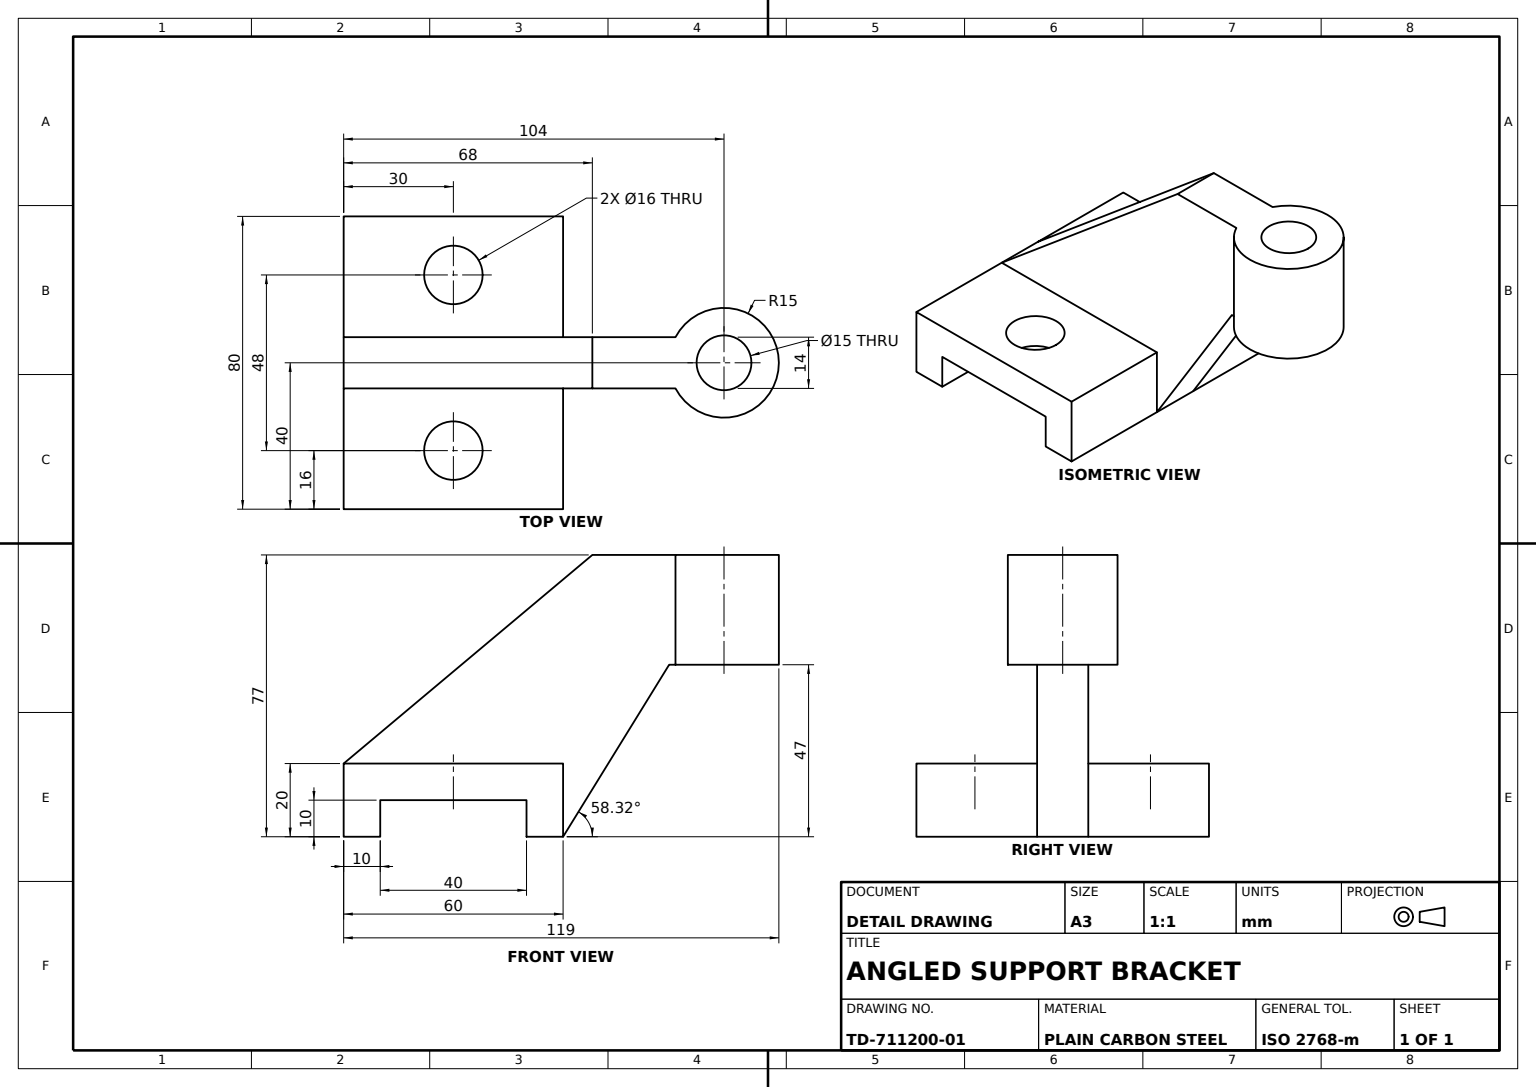
from build123d import *

# Parameters (mm, degrees)
BASE_PROFILE_SKETCH_W = 80
BASE_PROFILE_SKETCH_H = 20
BASE_BLOCK_DEPTH      = 30
ROUND_START           = 57
ROUND_BOSS_SKETCH_R   = 15
ROUND_BOSS_SKETCH_R_2 = 7.5
ROUND_BOSS_DEPTH      = 30
INCLINED_ARM_DEPTH    = 7
ARM_WEB_SKETCH_W      = 14
ARM_WEB_SKETCH_H      = 30
ARM_WEB_DEPTH         = 7
BASE_SLOT_SKETCH_W    = 40
BASE_SLOT_SKETCH_H    = 10
BASE_SLOT_40X10_DEPTH = 138.149553408
HOLE_CUT_SKETCH_R     = 8
HOLES_16_DEPTH        = 114.004424692


with BuildPart() as part:
    # Base Profile Sketch → Base Block (new, symmetric)
    with BuildSketch(Plane.XY):
        Rectangle(BASE_PROFILE_SKETCH_W, BASE_PROFILE_SKETCH_H)
    extrude(amount=BASE_BLOCK_DEPTH, both=True)

    # Inclined Arm Sketch → Inclined Arm (add, symmetric)
    with BuildSketch(Plane(origin=(0, 0, 0), x_dir=(0, 0, -1), z_dir=(1, 0, 0))):
        Polygon((-30, 10), (38, 67), (59, 67), (59, 37), (30, -10), (30, 10), align=None)
    extrude(amount=INCLINED_ARM_DEPTH, both=True)



with BuildPart() as body_2:
    # Round Boss Sketch → Round Boss (new body)
    with BuildSketch(Plane(origin=(0, 10, 0), x_dir=(1, 0, 0), z_dir=(0, 1, 0)).offset(ROUND_START)):
        with Locations(Location((0, 74, 0), (0, 0, 270))):
            Circle(ROUND_BOSS_SKETCH_R)
        with Locations(Location((0, 74, 0), (0, 0, 270))):
            Circle(ROUND_BOSS_SKETCH_R_2, mode=Mode.SUBTRACT)
    extrude(amount=-ROUND_BOSS_DEPTH)


with BuildPart() as part_1:
    add(part.part)

    add(body_2.part)  # Arm Web merges body 2
    # Arm Web Sketch → Arm Web (add, symmetric)
    with BuildSketch(Plane(origin=(0, 0, -59), x_dir=(-1, 0, 0), z_dir=(0, 0, -1))):
        with Locations((0, 52)):
            Rectangle(ARM_WEB_SKETCH_W, ARM_WEB_SKETCH_H)
    extrude(amount=ARM_WEB_DEPTH, both=True)

    # Base Slot Sketch → Base Slot 40x10 (cut, through all)
    with BuildSketch(Plane(origin=(40, 0, 0), x_dir=(0, 0, -1), z_dir=(1, 0, 0))):
        with Locations((0, -5)):
            Rectangle(BASE_SLOT_SKETCH_W, BASE_SLOT_SKETCH_H)
    extrude(amount=-BASE_SLOT_40X10_DEPTH, mode=Mode.SUBTRACT)

    # Hole Cut Sketch → Holes Ø16 (cut, through all)
    with BuildSketch(Plane(origin=(0, 10, 0), x_dir=(1, 0, 0), z_dir=(0, 1, 0))):
        with Locations(Location((-24, 0, 0), (0, 0, 270))):
            Circle(HOLE_CUT_SKETCH_R)
        with Locations(Location((24, 0, 0), (0, 0, 270))):
            Circle(HOLE_CUT_SKETCH_R)
    extrude(amount=-HOLES_16_DEPTH, mode=Mode.SUBTRACT)


solid = part_1.part
